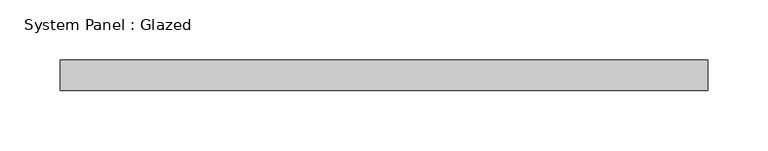
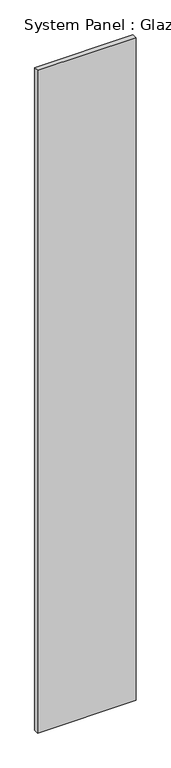
"""IFC4 building model written with IfcOpenShell, lengths in millimetres: plate geometry, System Panel : Glazed."""

from ifc_helpers import new_model, si_unit, origin, origin_with_axes, place, context, project, spatial, polyline, outline, extrude, source, transform, mapped, element, save


def system_panel_glazed_16a45962(model_context):
    return source(origin(), model_context, "Body", "SweptSolid", [
        extrude(outline(polyline([(269.7136875, 19.05), (-269.7136875, 19.05), (-269.7136875, 44.45), (269.7136875, 44.45), (269.7136875, 19.05)])), origin_with_axes(), (0.0, 0.0, 1.0), 3835.4),
    ])


if __name__ == "__main__":
    model = new_model("IFC4")
    model_context = context("Model", 3, world=origin())
    ifc_project = project(units=[si_unit("LENGTHUNIT", "METRE", prefix="MILLI")], contexts=[model_context])
    site = spatial("IfcSite", under=ifc_project)
    building = spatial("IfcBuilding", under=site)
    placement = place(None, origin())
    system_panel_glazed_shape = system_panel_glazed_16a45962(model_context)
    element("IfcPlate", 1, ObjectType="System Panel : Glazed", at=placement, inside=building, context=model_context, shape_type="MappedRepresentation", body=[
        mapped(system_panel_glazed_shape, transform((0.0, 0.0, 0.0), x_axis=(1.0, 0.0, 0.0), y_axis=(0.0, 1.0, 0.0), z_axis=(0.0, 0.0, 1.0))),
    ])
    save(model, "model.ifc")

# Revit data of these elements
# Type "System Panel : Glazed"
#   Construction Type Id = "GSP4R"
#   Analytic Construction = "1/8 in Pilkington single glazing"
#   Visual Light Transmittance = 0.9
#   Solar Heat Gain Coefficient = 0.86
#   Heat Transfer Coefficient (U) = 1.18115 BTU/(h·ft²·°F)
# Element 1 (IfcPlate, "System Panel : Glazed")
#   Materials on its faces: "Glass"
# Materials
#   "Glass": class "Glass", colour RGB 0 128 192, transparency 0.75, Description = "Soda Lime Glass", Cost = 0
